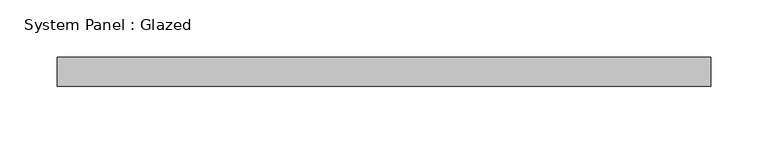
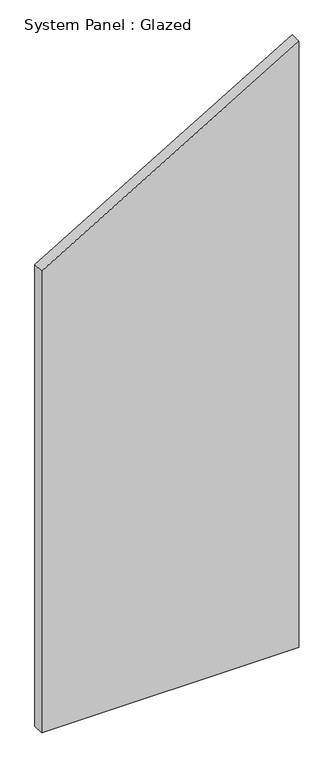
"""IFC4 building model written with IfcOpenShell, lengths in millimetres: plate geometry, System Panel : Glazed."""

from ifc_helpers import new_model, si_unit, frame, origin, place, context, project, spatial, polyline, outline, extrude, source, transform, mapped, element, save


def system_panel_glazed_ee2a426c(model_context):
    return source(origin(), model_context, "Body", "SweptSolid", [
        extrude(outline(polyline([(0.0, -285.75), (0.0, 285.75), (1424.9353958, 285.75), (1085.2676875, -285.75), (0.0, -285.75)])), frame((0.0, 19.05, 0.0), z_axis=(0.0, 1.0, 0.0), x_axis=(0.0, 0.0, 1.0)), (0.0, 0.0, 1.0), 25.4),
    ])


if __name__ == "__main__":
    model = new_model("IFC4")
    model_context = context("Model", 3, world=origin())
    ifc_project = project(units=[si_unit("LENGTHUNIT", "METRE", prefix="MILLI")], contexts=[model_context])
    site = spatial("IfcSite", under=ifc_project)
    building = spatial("IfcBuilding", under=site)
    placement = place(None, origin())
    system_panel_glazed_shape = system_panel_glazed_ee2a426c(model_context)
    element("IfcPlate", 1, ObjectType="System Panel : Glazed", at=placement, inside=building, context=model_context, shape_type="MappedRepresentation", body=[
        mapped(system_panel_glazed_shape, transform((0.0, 0.0, 0.0), x_axis=(1.0, 0.0, 0.0), y_axis=(0.0, 1.0, 0.0), z_axis=(0.0, 0.0, 1.0))),
    ])
    save(model, "model.ifc")

# Revit data of these elements
# Type "System Panel : Glazed"
#   Construction Type Id = "GSP4R"
#   Analytic Construction = "1/8 in Pilkington single glazing"
#   Visual Light Transmittance = 0.9
#   Solar Heat Gain Coefficient = 0.86
#   Heat Transfer Coefficient (U) = 1.18115 BTU/(h·ft²·°F)
#   Define Thermal Properties by = 1
# Element 1 (IfcPlate, "System Panel : Glazed")
#   Materials on its faces: "Glass"
# Materials
#   "Glass": class "Glass", colour RGB 0 128 192, transparency 0.75, Description = "Soda Lime Glass", Cost = 0
